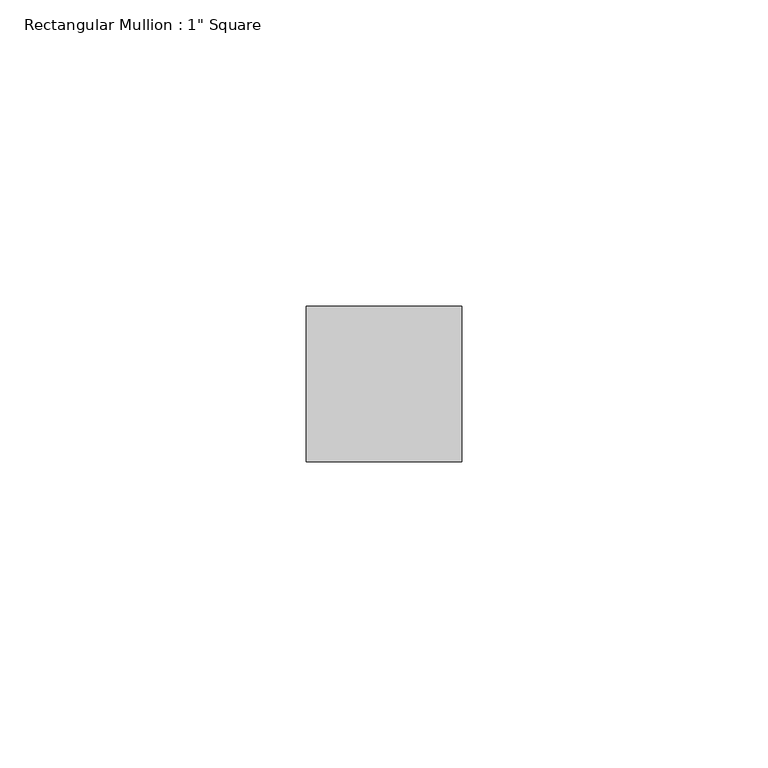
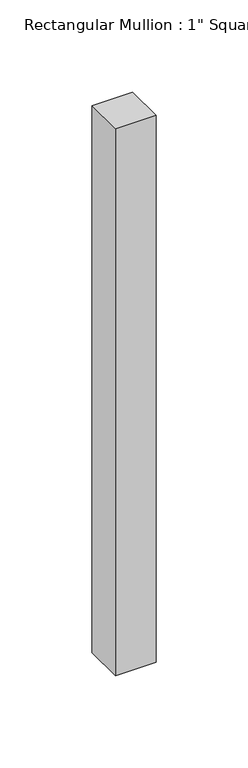
"""IFC4 building model written with IfcOpenShell, lengths in millimetres: member geometry."""

from ifc_helpers import new_model, si_unit, frame, origin, place, context, project, spatial, polyline, outline, extrude, source, transform, mapped, element, save


def member_2344d604(model_context):
    return source(origin(), model_context, "Body", "SweptSolid", [
        extrude(outline(polyline([(12.7, 12.7), (12.7, -12.7), (-12.7, -12.7), (-12.7, 12.7), (12.7, 12.7)])), frame((0.0, 0.0, -361.95), z_axis=(0.0, 0.0, 1.0), x_axis=(1.0, 0.0, 0.0)), (0.0, 0.0, 1.0), 361.95),
    ])


if __name__ == "__main__":
    model = new_model("IFC4")
    model_context = context("Model", 3, world=origin())
    ifc_project = project(units=[si_unit("LENGTHUNIT", "METRE", prefix="MILLI")], contexts=[model_context])
    site = spatial("IfcSite", under=ifc_project)
    building = spatial("IfcBuilding", under=site)
    placement = place(None, origin())
    member_shape = member_2344d604(model_context)
    element("IfcMember", 1, ObjectType="Rectangular Mullion : 1\" Square", at=placement, inside=building, context=model_context, shape_type="MappedRepresentation", body=[
        mapped(member_shape, transform((0.0, 0.0, 0.0), x_axis=(1.0, 0.0, 0.0), y_axis=(0.0, 1.0, 0.0), z_axis=(0.0, 0.0, 1.0))),
    ])
    save(model, "model.ifc")

# Revit data of these elements
# Type "Rectangular Mullion : 1\" Square"
#   built-in parameter 1007304 = 0.0833333 (stored number, unit not read)
#   built-in parameter 1007301 = 0.0416667 (stored number, unit not read)
#   built-in parameter 1007300 = 0.0416667 (stored number, unit not read)
